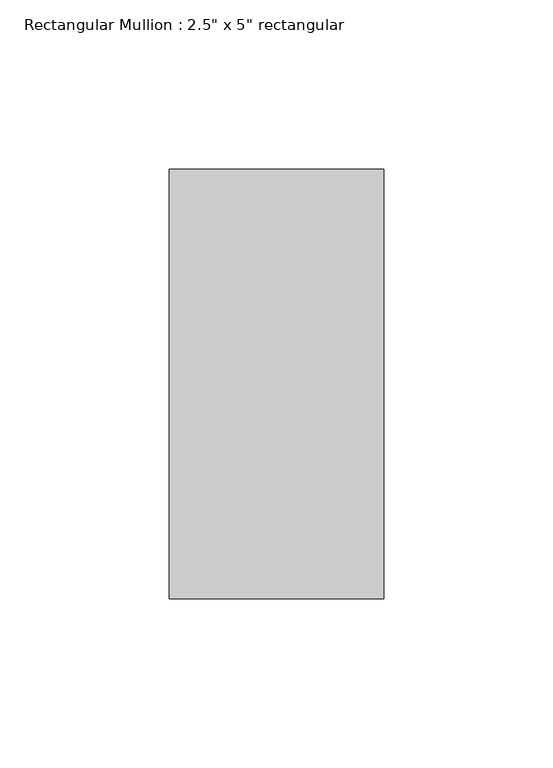
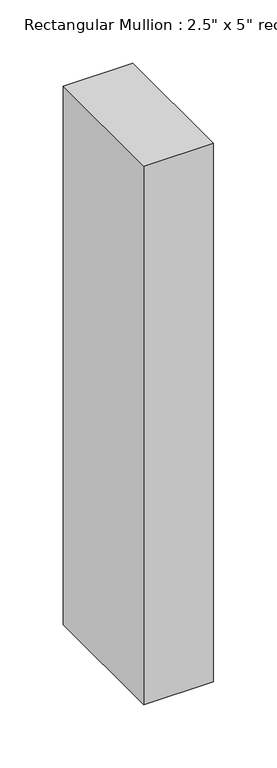
"""IFC4 building model written with IfcOpenShell, lengths in millimetres: member geometry."""

from ifc_helpers import new_model, si_unit, frame, origin, place, context, project, spatial, polyline, outline, extrude, source, transform, mapped, element, save


def member_6a4379ac(model_context):
    return source(origin(), model_context, "Body", "SweptSolid", [
        extrude(outline(polyline([(0.0, 63.5), (0.0, -63.5), (-63.5, -63.5), (-63.5, 63.5), (0.0, 63.5)])), frame((0.0, 0.0, -519.2098371), z_axis=(0.0, 0.0, 1.0), x_axis=(1.0, 0.0, 0.0)), (0.0, 0.0, 1.0), 519.2098371),
    ])


if __name__ == "__main__":
    model = new_model("IFC4")
    model_context = context("Model", 3, world=origin())
    ifc_project = project(units=[si_unit("LENGTHUNIT", "METRE", prefix="MILLI")], contexts=[model_context])
    site = spatial("IfcSite", under=ifc_project)
    building = spatial("IfcBuilding", under=site)
    placement = place(None, origin())
    member_shape = member_6a4379ac(model_context)
    element("IfcMember", 1, ObjectType="Rectangular Mullion : 2.5\" x 5\" rectangular", at=placement, inside=building, context=model_context, shape_type="MappedRepresentation", body=[
        mapped(member_shape, transform((0.0, 0.0, 0.0), x_axis=(1.0, 0.0, 0.0), y_axis=(0.0, 1.0, 0.0), z_axis=(0.0, 0.0, 1.0))),
    ])
    save(model, "model.ifc")

# Revit data of these elements
# Type "Rectangular Mullion : 2.5\" x 5\" rectangular"
#   built-in parameter 1007304 = 0.416667 (stored number, unit not read)
#   built-in parameter 1007301 = 0.104167 (stored number, unit not read)
#   built-in parameter 1007300 = 0.104167 (stored number, unit not read)
# Element 1 (IfcMember, "Rectangular Mullion : 2.5\" x 5\" rectangular")
#   Materials on its faces: "mullions"
# Materials
#   "mullions": class "Generic", colour RGB 120 120 120, transparency 0, Cost = 0
